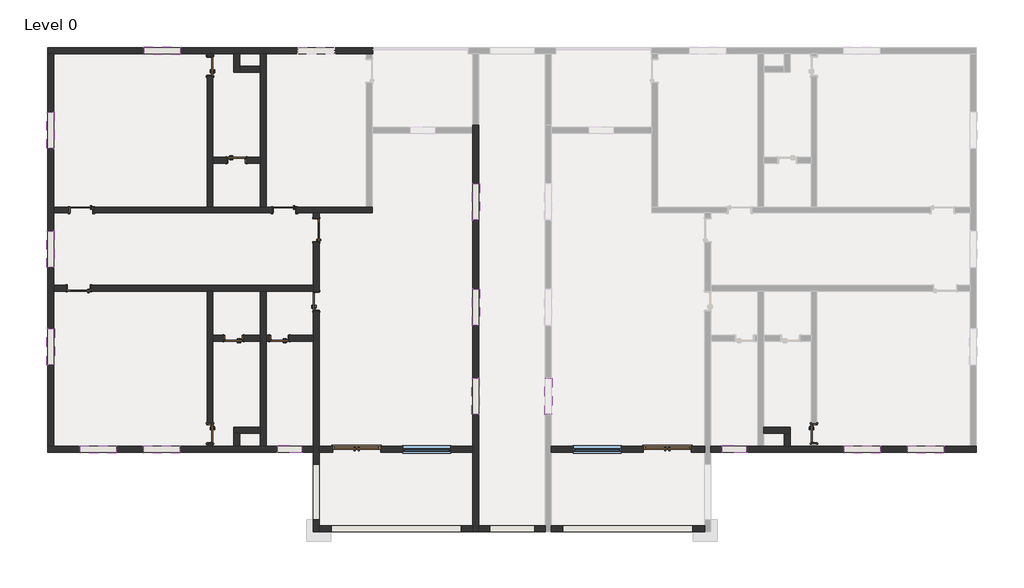
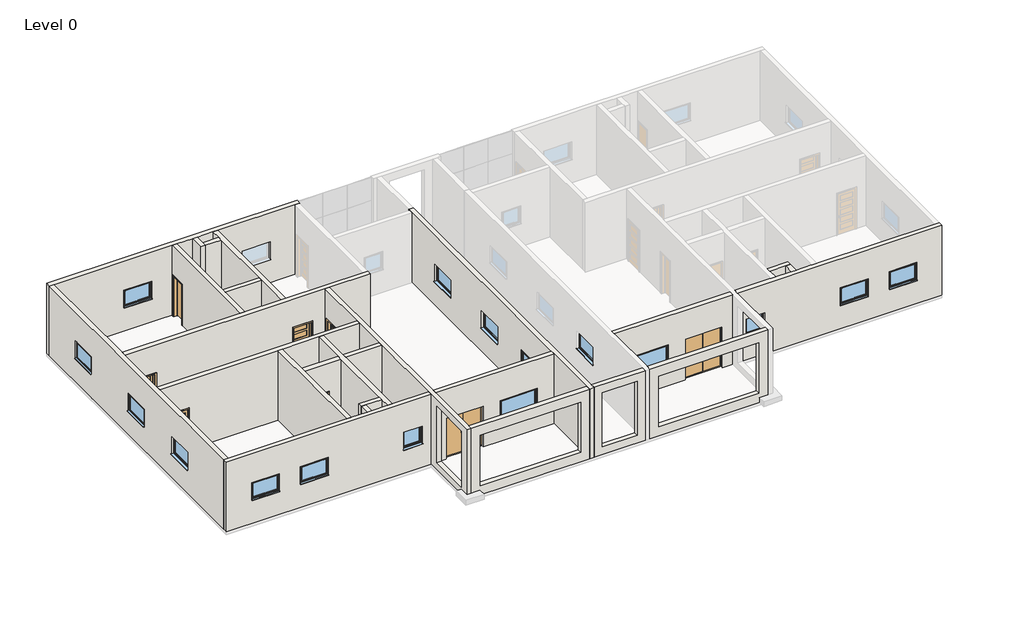
# One storey, part 1 of 2: 25 walls, 16 windows, 13 doors.
"""IFC4 building model written with IfcOpenShell, lengths in millimetres."""

from ifc_helpers import new_model, si_unit, frame, origin, origin_with_axes, place, context, project, spatial, polyline, outline, extrude, faceted_brep, transform, mapped, element, save
from components import door_interior_single_5_panel_vert_wood_door_interior_single_0f225555, door_interior_single_5_panel_vert_wood_door_interior_single_643f6a0b, doors_extdbl_flush_1810x2110mm_a954e790, doors_extdbl_flush_1810x2110mm_cf8af4c5, doors_intsgl_750x2110mm_542c0a28, doors_intsgl_750x2110mm_8b4efb5c, windows_sgl_plain_1360x910mm_f5b307ae, windows_sgl_plain_1360x910mm_8a2bb76a, windows_sgl_plain_1810x1210mm_77c2169a, windows_sgl_plain_1810x1210mm_541be4ad, windows_sgl_plain_910x910mm_7835b02d, windows_sgl_plain_910x910mm_23580505

model = new_model("IFC4")

# Units and contexts
model_context = context("Model", 3, world=origin())
ifc_project = project(units=[si_unit("LENGTHUNIT", "METRE", prefix="MILLI")], contexts=[model_context])

# Site, building, storey
site = spatial("IfcSite", under=ifc_project)
building = spatial("IfcBuilding", under=site)
storey = spatial("IfcBuildingStorey", under=building, Name="Level 0", Elevation=0.0)

# Doors
placement = place(None, origin())
door_interior_single_5_panel_vert_wood_door_interior_single_shape = door_interior_single_5_panel_vert_wood_door_interior_single_0f225555(model_context)
element("IfcDoor", 1, ObjectType="Door-Interior-Single-5_Panel_Vert-Wood : Door-Interior-Single-5_Panel_Vert-Wood", at=placement, inside=storey, context=model_context, shape_type="MappedRepresentation", body=[
    mapped(door_interior_single_5_panel_vert_wood_door_interior_single_shape, transform((-948.8269071, 3233.5358821, 0.0), x_axis=(-1.0, 0.0, 0.0), y_axis=(0.0, -1.0, 0.0), z_axis=(0.0, 0.0, 1.0))),
])
door_interior_single_5_panel_vert_wood_door_interior_single_2_shape = door_interior_single_5_panel_vert_wood_door_interior_single_643f6a0b(model_context)
element("IfcDoor", 2, ObjectType="Door-Interior-Single-5_Panel_Vert-Wood : Door-Interior-Single-5_Panel_Vert-Wood", at=placement, inside=storey, context=model_context, shape_type="MappedRepresentation", body=[
    mapped(door_interior_single_5_panel_vert_wood_door_interior_single_2_shape, transform((6788.6730929, 6189.8858821, 0.0), x_axis=(-1.0, 0.0, 0.0), y_axis=(0.0, -1.0, 0.0), z_axis=(0.0, 0.0, 1.0))),
])
element("IfcDoor", 3, ObjectType="Door-Interior-Single-5_Panel_Vert-Wood : Door-Interior-Single-5_Panel_Vert-Wood", at=placement, inside=storey, context=model_context, shape_type="MappedRepresentation", body=[
    mapped(door_interior_single_5_panel_vert_wood_door_interior_single_2_shape, transform((-848.8269071, 6189.8858821, 0.0), x_axis=(-1.0, 0.0, 0.0), y_axis=(0.0, -1.0, 0.0), z_axis=(0.0, 0.0, 1.0))),
])
element("IfcDoor", 4, ObjectType="Door-Interior-Single-5_Panel_Vert-Wood : Door-Interior-Single-5_Panel_Vert-Wood", at=placement, inside=storey, context=model_context, shape_type="MappedRepresentation", body=[
    mapped(door_interior_single_5_panel_vert_wood_door_interior_single_2_shape, transform((7991.8480929, 5424.2108821, 0.0), x_axis=(0.0, 1.0, 0.0), y_axis=(-1.0, 0.0, 0.0), z_axis=(0.0, 0.0, 1.0))),
])
doors_extdbl_flush_1810x2110mm_shape = doors_extdbl_flush_1810x2110mm_a954e790(model_context)
element("IfcDoor", 5, ObjectType="Doors_ExtDbl_Flush : 1810x2110mm", at=placement, inside=storey, context=model_context, shape_type="MappedRepresentation", body=[
    mapped(doors_extdbl_flush_1810x2110mm_shape, transform((9506.1730929, -2813.2891179, 0.0), x_axis=(1.0, 0.0, 0.0), y_axis=(0.0, 1.0, 0.0), z_axis=(0.0, 0.0, 1.0))),
])
doors_extdbl_flush_1810x2110mm_2_shape = doors_extdbl_flush_1810x2110mm_cf8af4c5(model_context)
element("IfcDoor", 6, ObjectType="Doors_ExtDbl_Flush : 1810x2110mm", at=placement, inside=storey, context=model_context, shape_type="MappedRepresentation", body=[
    mapped(doors_extdbl_flush_1810x2110mm_2_shape, transform((21196.1730929, -2813.2891179, 0.0), x_axis=(-1.0, 0.0, 0.0), y_axis=(0.0, -1.0, 0.0), z_axis=(0.0, 0.0, 1.0))),
])
doors_intsgl_750x2110mm_shape = doors_intsgl_750x2110mm_542c0a28(model_context)
element("IfcDoor", 7, ObjectType="Doors_IntSgl : 750x2110mm", at=placement, inside=storey, context=model_context, shape_type="MappedRepresentation", body=[
    mapped(doors_intsgl_750x2110mm_shape, transform((4988.6730929, 8061.7108821, 0.0), x_axis=(1.0, 0.0, 0.0), y_axis=(0.0, 1.0, 0.0), z_axis=(0.0, 0.0, 1.0))),
])
element("IfcDoor", 8, ObjectType="Doors_IntSgl : 750x2110mm", at=placement, inside=storey, context=model_context, shape_type="MappedRepresentation", body=[
    mapped(doors_intsgl_750x2110mm_shape, transform((4876.1730929, 1361.7108821, 0.0), x_axis=(-1.0, 0.0, 0.0), y_axis=(0.0, -1.0, 0.0), z_axis=(0.0, 0.0, 1.0))),
])
element("IfcDoor", 9, ObjectType="Doors_IntSgl : 750x2110mm", at=placement, inside=storey, context=model_context, shape_type="MappedRepresentation", body=[
    mapped(doors_intsgl_750x2110mm_shape, transform((6601.1730929, 1361.7108821, 0.0), x_axis=(-1.0, 0.0, 0.0), y_axis=(0.0, -1.0, 0.0), z_axis=(0.0, 0.0, 1.0))),
])
element("IfcDoor", 10, ObjectType="Doors_IntSgl : 750x2110mm", at=placement, inside=storey, context=model_context, shape_type="MappedRepresentation", body=[
    mapped(doors_intsgl_750x2110mm_shape, transform((7988.6730929, 2749.2108821, 0.0), x_axis=(0.0, 1.0, 0.0), y_axis=(-1.0, 0.0, 0.0), z_axis=(0.0, 0.0, 1.0))),
])
element("IfcDoor", 11, ObjectType="Doors_IntSgl : 750x2110mm", at=placement, inside=storey, context=model_context, shape_type="MappedRepresentation", body=[
    mapped(doors_intsgl_750x2110mm_shape, transform((3988.6730929, -2225.7891179, 0.0), x_axis=(0.0, -1.0, 0.0), y_axis=(1.0, 0.0, 0.0), z_axis=(0.0, 0.0, 1.0))),
])
doors_intsgl_750x2110mm_2_shape = doors_intsgl_750x2110mm_8b4efb5c(model_context)
element("IfcDoor", 12, ObjectType="Doors_IntSgl : 750x2110mm", at=placement, inside=storey, context=model_context, shape_type="MappedRepresentation", body=[
    mapped(doors_intsgl_750x2110mm_2_shape, transform((3988.6730929, 11599.2108821, 0.0), x_axis=(0.0, 1.0, 0.0), y_axis=(-1.0, 0.0, 0.0), z_axis=(0.0, 0.0, 1.0))),
])
element("IfcDoor", 13, ObjectType="Doors_IntSgl : 750x2110mm", at=placement, inside=storey, context=model_context, shape_type="MappedRepresentation", body=[
    mapped(doors_intsgl_750x2110mm_2_shape, transform((26713.6730929, -2225.7891179, 0.0), x_axis=(0.0, -1.0, 0.0), y_axis=(1.0, 0.0, 0.0), z_axis=(0.0, 0.0, 1.0))),
])

# Walls
element("IfcWall", 14, ObjectType="GENERIC 225", at=placement, inside=storey, context=model_context, shape_type="Brep", body=[
    faceted_brep([(-2123.8269071, 12074.2108821, 0.0), (-1898.8269071, 12074.2108821, 0.0), (3876.1730929, 12074.2108821, 0.0), (4101.1730929, 12074.2108821, 0.0), (4876.1730929, 12074.2108821, 0.0), (5101.1730929, 12074.2108821, 0.0), (5876.1730929, 12074.2108821, 0.0), (6101.1730929, 12074.2108821, 0.0), (9876.1730929, 12074.2108821, 0.0), (10101.1730929, 12074.2108821, 0.0), (10121.1730929, 12074.2108821, 0.0), (10121.1730929, 12074.2108821, 3600.0), (10101.1730929, 12074.2108821, 3600.0), (9876.1730929, 12074.2108821, 3600.0), (6101.1730929, 12074.2108821, 3600.0), (5876.1730929, 12074.2108821, 3600.0), (5101.1730929, 12074.2108821, 3600.0), (4876.1730929, 12074.2108821, 3600.0), (4101.1730929, 12074.2108821, 3600.0), (3876.1730929, 12074.2108821, 3600.0), (-1898.8269071, 12074.2108821, 3600.0), (-2123.8269071, 12074.2108821, 3600.0), (2876.1730929, 12074.2108821, 2110.0), (2876.1730929, 12074.2108821, 1200.0), (1516.1730929, 12074.2108821, 1200.0), (1516.1730929, 12074.2108821, 2110.0), (7308.6730929, 12074.2108821, 2110.0), (8668.6730929, 12074.2108821, 2110.0), (8668.6730929, 12074.2108821, 1200.0), (7308.6730929, 12074.2108821, 1200.0), (-2123.8269071, 12299.2108821, 0.0), (-2123.8269071, 12299.2108821, 3600.0), (10121.1730929, 12299.2108821, 3600.0), (10121.1730929, 12299.2108821, 0.0), (2876.1730929, 12299.2108821, 2110.0), (1516.1730929, 12299.2108821, 2110.0), (1516.1730929, 12299.2108821, 1200.0), (2876.1730929, 12299.2108821, 1200.0), (7308.6730929, 12299.2108821, 2110.0), (7308.6730929, 12299.2108821, 1200.0), (8668.6730929, 12299.2108821, 1200.0), (8668.6730929, 12299.2108821, 2110.0)], [[[0, 1, 2, 3, 4, 5, 6, 7, 8, 9, 10, 11, 12, 13, 14, 15, 16, 17, 18, 19, 20, 21], [22, 23, 24, 25], [26, 27, 28, 29]], [[30, 31, 32, 33], [34, 35, 36, 37], [38, 39, 40, 41]], [[10, 9, 8, 7, 6, 5, 4, 3, 2, 1, 0, 30, 33]], [[11, 10, 33, 32]], [[21, 20, 19, 18, 17, 16, 15, 14, 13, 12, 11, 32, 31]], [[0, 21, 31, 30]], [[23, 22, 34, 37]], [[24, 23, 37, 36]], [[25, 24, 36, 35]], [[22, 25, 35, 34]], [[39, 38, 26, 29]], [[40, 39, 29, 28]], [[41, 40, 28, 27]], [[38, 41, 27, 26]]]),
])
element("IfcWall", 15, ObjectType="GENERIC 225", at=placement, inside=storey, context=model_context, shape_type="Brep", body=[
    faceted_brep([(8101.1730929, 6074.2108821, 3600.0), (8101.1730929, -2700.7891179, 3600.0), (8101.1730929, -2925.7891179, 3600.0), (8101.1730929, -5700.7891179, 3600.0), (8101.1730929, -5925.7891179, 3600.0), (8101.1730929, -5925.7891179, 0.0), (8101.1730929, -5700.7891179, 0.0), (8101.1730929, -2925.7891179, 0.0), (8101.1730929, -2700.7891179, 0.0), (8101.1730929, 2374.2108821, 0.0), (8101.1730929, 2374.2108821, 2110.0), (8101.1730929, 3124.2108821, 2110.0), (8101.1730929, 3124.2108821, 0.0), (8101.1730929, 4974.2108821, 0.0), (8101.1730929, 4974.2108821, 2125.4), (8101.1730929, 5874.2108821, 2125.4), (8101.1730929, 5874.2108821, 0.0), (8101.1730929, 6074.2108821, 0.0), (8101.1730929, -5475.2269163, 3254.1937526), (8101.1730929, -3375.2269163, 3254.1937526), (8101.1730929, -3375.2269163, 354.1937526), (8101.1730929, -5475.2269163, 354.1937526), (7876.1730929, -5925.7891179, 3600.0), (7876.1730929, -2925.7891179, 3600.0), (7876.1730929, -2700.7891179, 3600.0), (7876.1730929, 1249.2108821, 3600.0), (7876.1730929, 1474.2108821, 3600.0), (7876.1730929, 3124.2108821, 3600.0), (7876.1730929, 3349.2108821, 3600.0), (7876.1730929, 6074.2108821, 3600.0), (7876.1730929, 6074.2108821, 0.0), (7876.1730929, 5874.2108821, 0.0), (7876.1730929, 5874.2108821, 2125.4), (7876.1730929, 4974.2108821, 2125.4), (7876.1730929, 4974.2108821, 0.0), (7876.1730929, 3349.2108821, 0.0), (7876.1730929, 3124.2108821, 0.0), (7876.1730929, 3124.2108821, 2110.0), (7876.1730929, 2374.2108821, 2110.0), (7876.1730929, 2374.2108821, 0.0), (7876.1730929, 1474.2108821, 0.0), (7876.1730929, 1249.2108821, 0.0), (7876.1730929, -2700.7891179, 0.0), (7876.1730929, -2925.7891179, 0.0), (7876.1730929, -5925.7891179, 0.0), (7876.1730929, -3375.2269163, 3254.1937526), (7876.1730929, -5475.2269163, 3254.1937526), (7876.1730929, -5475.2269163, 354.1937526), (7876.1730929, -3375.2269163, 354.1937526)], [[[0, 1, 2, 3, 4, 5, 6, 7, 8, 9, 10, 11, 12, 13, 14, 15, 16, 17], [18, 19, 20, 21]], [[22, 23, 24, 25, 26, 27, 28, 29, 30, 31, 32, 33, 34, 35, 36, 37, 38, 39, 40, 41, 42, 43, 44], [45, 46, 47, 48]], [[0, 17, 30, 29]], [[15, 32, 31, 16]], [[32, 15, 14, 33]], [[33, 14, 13, 34]], [[11, 37, 36, 12]], [[37, 11, 10, 38]], [[38, 10, 9, 39]], [[5, 4, 22, 44]], [[17, 16, 31, 30]], [[5, 44, 43, 42, 41, 40, 39, 9, 8, 7, 6]], [[34, 13, 12, 36, 35]], [[4, 3, 2, 1, 0, 29, 28, 27, 26, 25, 24, 23, 22]], [[19, 18, 46, 45]], [[20, 19, 45, 48]], [[21, 20, 48, 47]], [[18, 21, 47, 46]]]),
])
element("IfcWall", 16, ObjectType="GENERIC 225", at=placement, inside=storey, context=model_context, shape_type="Brep", body=[
    faceted_brep([(7876.1730929, -2700.7891179, 0.0), (6101.1730929, -2700.7891179, 0.0), (5876.1730929, -2700.7891179, 0.0), (5101.1730929, -2700.7891179, 0.0), (4876.1730929, -2700.7891179, 0.0), (4101.1730929, -2700.7891179, 0.0), (3876.1730929, -2700.7891179, 0.0), (-1898.8269071, -2700.7891179, 0.0), (-2123.8269071, -2700.7891179, 0.0), (-2123.8269071, -2700.7891179, 3600.0), (-1898.8269071, -2700.7891179, 3600.0), (3876.1730929, -2700.7891179, 3600.0), (4101.1730929, -2700.7891179, 3600.0), (4876.1730929, -2700.7891179, 3600.0), (5101.1730929, -2700.7891179, 3600.0), (5876.1730929, -2700.7891179, 3600.0), (6101.1730929, -2700.7891179, 3600.0), (7876.1730929, -2700.7891179, 3600.0), (461.1730929, -2700.7891179, 2110.0), (-898.8269071, -2700.7891179, 2110.0), (-898.8269071, -2700.7891179, 1200.0), (461.1730929, -2700.7891179, 1200.0), (2848.6730929, -2700.7891179, 2110.0), (1488.6730929, -2700.7891179, 2110.0), (1488.6730929, -2700.7891179, 1200.0), (2848.6730929, -2700.7891179, 1200.0), (6533.6730929, -2700.7891179, 2110.0), (6533.6730929, -2700.7891179, 1200.0), (7443.6730929, -2700.7891179, 1200.0), (7443.6730929, -2700.7891179, 2110.0), (7876.1730929, -2925.7891179, 0.0), (7876.1730929, -2925.7891179, 3600.0), (-2123.8269071, -2925.7891179, 3600.0), (-2123.8269071, -2925.7891179, 0.0), (461.1730929, -2925.7891179, 2110.0), (461.1730929, -2925.7891179, 1200.0), (-898.8269071, -2925.7891179, 1200.0), (-898.8269071, -2925.7891179, 2110.0), (2848.6730929, -2925.7891179, 2110.0), (2848.6730929, -2925.7891179, 1200.0), (1488.6730929, -2925.7891179, 1200.0), (1488.6730929, -2925.7891179, 2110.0), (6533.6730929, -2925.7891179, 2110.0), (7443.6730929, -2925.7891179, 2110.0), (7443.6730929, -2925.7891179, 1200.0), (6533.6730929, -2925.7891179, 1200.0)], [[[0, 1, 2, 3, 4, 5, 6, 7, 8, 9, 10, 11, 12, 13, 14, 15, 16, 17], [18, 19, 20, 21], [22, 23, 24, 25], [26, 27, 28, 29]], [[30, 31, 32, 33], [34, 35, 36, 37], [38, 39, 40, 41], [42, 43, 44, 45]], [[8, 7, 6, 5, 4, 3, 2, 1, 0, 30, 33]], [[17, 16, 15, 14, 13, 12, 11, 10, 9, 32, 31]], [[0, 17, 31, 30]], [[9, 8, 33, 32]], [[35, 34, 18, 21]], [[36, 35, 21, 20]], [[37, 36, 20, 19]], [[34, 37, 19, 18]], [[39, 38, 22, 25]], [[40, 39, 25, 24]], [[41, 40, 24, 23]], [[38, 41, 23, 22]], [[27, 26, 42, 45]], [[28, 27, 45, 44]], [[29, 28, 44, 43]], [[26, 29, 43, 42]]]),
])
element("IfcWall", 17, ObjectType="GENERIC 225", at=placement, inside=storey, context=model_context, shape_type="Brep", body=[
    faceted_brep([(-1898.8269071, -2700.7891179, 0.0), (-1898.8269071, 3124.2108821, 0.0), (-1898.8269071, 3349.2108821, 0.0), (-1898.8269071, 6074.2108821, 0.0), (-1898.8269071, 6299.2108821, 0.0), (-1898.8269071, 12074.2108821, 0.0), (-1898.8269071, 12074.2108821, 3600.0), (-1898.8269071, 6299.2108821, 3600.0), (-1898.8269071, 6074.2108821, 3600.0), (-1898.8269071, 3349.2108821, 3600.0), (-1898.8269071, 3124.2108821, 3600.0), (-1898.8269071, -2700.7891179, 3600.0), (-1898.8269071, 8506.7108821, 2110.0), (-1898.8269071, 9866.7108821, 2110.0), (-1898.8269071, 9866.7108821, 1200.0), (-1898.8269071, 8506.7108821, 1200.0), (-1898.8269071, 4031.7108821, 2110.0), (-1898.8269071, 5391.7108821, 2110.0), (-1898.8269071, 5391.7108821, 1200.0), (-1898.8269071, 4031.7108821, 1200.0), (-1898.8269071, 1724.2108821, 2110.0), (-1898.8269071, 1724.2108821, 1200.0), (-1898.8269071, 364.2108821, 1200.0), (-1898.8269071, 364.2108821, 2110.0), (-2123.8269071, -2700.7891179, 0.0), (-2123.8269071, -2700.7891179, 3600.0), (-2123.8269071, 12074.2108821, 3600.0), (-2123.8269071, 12074.2108821, 0.0), (-2123.8269071, 8506.7108821, 2110.0), (-2123.8269071, 8506.7108821, 1200.0), (-2123.8269071, 9866.7108821, 1200.0), (-2123.8269071, 9866.7108821, 2110.0), (-2123.8269071, 4031.7108821, 2110.0), (-2123.8269071, 4031.7108821, 1200.0), (-2123.8269071, 5391.7108821, 1200.0), (-2123.8269071, 5391.7108821, 2110.0), (-2123.8269071, 1724.2108821, 2110.0), (-2123.8269071, 364.2108821, 2110.0), (-2123.8269071, 364.2108821, 1200.0), (-2123.8269071, 1724.2108821, 1200.0)], [[[0, 1, 2, 3, 4, 5, 6, 7, 8, 9, 10, 11], [12, 13, 14, 15], [16, 17, 18, 19], [20, 21, 22, 23]], [[24, 25, 26, 27], [28, 29, 30, 31], [32, 33, 34, 35], [36, 37, 38, 39]], [[5, 4, 3, 2, 1, 0, 24, 27]], [[11, 10, 9, 8, 7, 6, 26, 25]], [[6, 5, 27, 26]], [[0, 11, 25, 24]], [[29, 28, 12, 15]], [[30, 29, 15, 14]], [[31, 30, 14, 13]], [[28, 31, 13, 12]], [[33, 32, 16, 19]], [[34, 33, 19, 18]], [[35, 34, 18, 17]], [[32, 35, 17, 16]], [[21, 20, 36, 39]], [[22, 21, 39, 38]], [[23, 22, 38, 37]], [[20, 23, 37, 36]]]),
])
element("IfcWall", 18, ObjectType="GENERIC 225", at=placement, inside=storey, context=model_context, shape_type="Brep", body=[
    faceted_brep([(7876.1730929, 3124.2108821, 3600.0), (6101.1730929, 3124.2108821, 3600.0), (5876.1730929, 3124.2108821, 3600.0), (4101.1730929, 3124.2108821, 3600.0), (3876.1730929, 3124.2108821, 3600.0), (-1898.8269071, 3124.2108821, 3600.0), (-1898.8269071, 3124.2108821, 0.0), (-1398.8269071, 3124.2108821, 0.0), (-1398.8269071, 3124.2108821, 2125.4), (-498.8269071, 3124.2108821, 2125.4), (-498.8269071, 3124.2108821, 0.0), (3876.1730929, 3124.2108821, 0.0), (4101.1730929, 3124.2108821, 0.0), (5876.1730929, 3124.2108821, 0.0), (6101.1730929, 3124.2108821, 0.0), (7876.1730929, 3124.2108821, 0.0), (7876.1730929, 3124.2108821, 2110.0), (-1898.8269071, 3349.2108821, 3600.0), (7876.1730929, 3349.2108821, 3600.0), (7876.1730929, 3349.2108821, 0.0), (-498.8269071, 3349.2108821, 0.0), (-498.8269071, 3349.2108821, 2125.4), (-1398.8269071, 3349.2108821, 2125.4), (-1398.8269071, 3349.2108821, 0.0), (-1898.8269071, 3349.2108821, 0.0)], [[[0, 1, 2, 3, 4, 5, 6, 7, 8, 9, 10, 11, 12, 13, 14, 15, 16]], [[17, 18, 19, 20, 21, 22, 23, 24]], [[6, 24, 23, 7]], [[19, 15, 14, 13, 12, 11, 10, 20]], [[5, 4, 3, 2, 1, 0, 18, 17]], [[6, 5, 17, 24]], [[0, 16, 15, 19, 18]], [[22, 8, 7, 23]], [[8, 22, 21, 9]], [[9, 21, 20, 10]]]),
])
element("IfcWall", 19, ObjectType="GENERIC 225", at=placement, inside=storey, context=model_context, shape_type="Brep", body=[
    faceted_brep([(3876.1730929, -2700.7891179, 3600.0), (3876.1730929, 3124.2108821, 3600.0), (3876.1730929, 3124.2108821, 0.0), (3876.1730929, -1850.7891179, 0.0), (3876.1730929, -1850.7891179, 2110.0), (3876.1730929, -2600.7891179, 2110.0), (3876.1730929, -2600.7891179, 0.0), (3876.1730929, -2700.7891179, 0.0), (4101.1730929, 3124.2108821, 3600.0), (4101.1730929, 1474.2108821, 3600.0), (4101.1730929, 1249.2108821, 3600.0), (4101.1730929, -2700.7891179, 3600.0), (4101.1730929, -2700.7891179, 0.0), (4101.1730929, -2600.7891179, 0.0), (4101.1730929, -2600.7891179, 2110.0), (4101.1730929, -1850.7891179, 2110.0), (4101.1730929, -1850.7891179, 0.0), (4101.1730929, 1249.2108821, 0.0), (4101.1730929, 1474.2108821, 0.0), (4101.1730929, 3124.2108821, 0.0)], [[[0, 1, 2, 3, 4, 5, 6, 7]], [[8, 9, 10, 11, 12, 13, 14, 15, 16, 17, 18, 19]], [[2, 19, 18, 17, 16, 3]], [[12, 7, 6, 13]], [[1, 0, 11, 10, 9, 8]], [[2, 1, 8, 19]], [[0, 7, 12, 11]], [[5, 14, 13, 6]], [[14, 5, 4, 15]], [[15, 4, 3, 16]]]),
])
element("IfcWall", 20, ObjectType="GENERIC 225", at=placement, inside=storey, context=model_context, shape_type="Brep", body=[
    faceted_brep([(10101.1730929, 6074.2108821, 3600.0), (8101.1730929, 6074.2108821, 3600.0), (7876.1730929, 6074.2108821, 3600.0), (-1898.8269071, 6074.2108821, 3600.0), (-1898.8269071, 6074.2108821, 0.0), (-1298.8269071, 6074.2108821, 0.0), (-1298.8269071, 6074.2108821, 2125.4), (-398.8269071, 6074.2108821, 2125.4), (-398.8269071, 6074.2108821, 0.0), (6338.6730929, 6074.2108821, 0.0), (6338.6730929, 6074.2108821, 2125.4), (7238.6730929, 6074.2108821, 2125.4), (7238.6730929, 6074.2108821, 0.0), (7876.1730929, 6074.2108821, 0.0), (8101.1730929, 6074.2108821, 0.0), (10101.1730929, 6074.2108821, 0.0), (-1898.8269071, 6299.2108821, 3600.0), (3876.1730929, 6299.2108821, 3600.0), (4101.1730929, 6299.2108821, 3600.0), (5876.1730929, 6299.2108821, 3600.0), (6101.1730929, 6299.2108821, 3600.0), (9876.1730929, 6299.2108821, 3600.0), (10101.1730929, 6299.2108821, 3600.0), (10101.1730929, 6299.2108821, 0.0), (9876.1730929, 6299.2108821, 0.0), (7238.6730929, 6299.2108821, 0.0), (7238.6730929, 6299.2108821, 2125.4), (6338.6730929, 6299.2108821, 2125.4), (6338.6730929, 6299.2108821, 0.0), (6101.1730929, 6299.2108821, 0.0), (5876.1730929, 6299.2108821, 0.0), (4101.1730929, 6299.2108821, 0.0), (3876.1730929, 6299.2108821, 0.0), (-398.8269071, 6299.2108821, 0.0), (-398.8269071, 6299.2108821, 2125.4), (-1298.8269071, 6299.2108821, 2125.4), (-1298.8269071, 6299.2108821, 0.0), (-1898.8269071, 6299.2108821, 0.0)], [[[0, 1, 2, 3, 4, 5, 6, 7, 8, 9, 10, 11, 12, 13, 14, 15]], [[16, 17, 18, 19, 20, 21, 22, 23, 24, 25, 26, 27, 28, 29, 30, 31, 32, 33, 34, 35, 36, 37]], [[4, 37, 36, 5]], [[23, 15, 14, 13, 12, 25, 24]], [[28, 9, 8, 33, 32, 31, 30, 29]], [[3, 2, 1, 0, 22, 21, 20, 19, 18, 17, 16]], [[4, 3, 16, 37]], [[0, 15, 23, 22]], [[10, 9, 28, 27]], [[11, 10, 27, 26]], [[12, 11, 26, 25]], [[35, 6, 5, 36]], [[6, 35, 34, 7]], [[7, 34, 33, 8]]]),
])
element("IfcWall", 21, ObjectType="GENERIC 225", at=placement, inside=storey, context=model_context, shape_type="Brep", body=[
    faceted_brep([(4101.1730929, 12074.2108821, 3600.0), (4101.1730929, 8174.2108821, 3600.0), (4101.1730929, 7949.2108821, 3600.0), (4101.1730929, 6299.2108821, 3600.0), (4101.1730929, 6299.2108821, 0.0), (4101.1730929, 7949.2108821, 0.0), (4101.1730929, 8174.2108821, 0.0), (4101.1730929, 11224.2108821, 0.0), (4101.1730929, 11224.2108821, 2110.0), (4101.1730929, 11974.2108821, 2110.0), (4101.1730929, 11974.2108821, 0.0), (4101.1730929, 12074.2108821, 0.0), (3876.1730929, 6299.2108821, 3600.0), (3876.1730929, 12074.2108821, 3600.0), (3876.1730929, 12074.2108821, 0.0), (3876.1730929, 11974.2108821, 0.0), (3876.1730929, 11974.2108821, 2110.0), (3876.1730929, 11224.2108821, 2110.0), (3876.1730929, 11224.2108821, 0.0), (3876.1730929, 6299.2108821, 0.0)], [[[0, 1, 2, 3, 4, 5, 6, 7, 8, 9, 10, 11]], [[12, 13, 14, 15, 16, 17, 18, 19]], [[4, 19, 18, 7, 6, 5]], [[14, 11, 10, 15]], [[3, 2, 1, 0, 13, 12]], [[4, 3, 12, 19]], [[0, 11, 14, 13]], [[9, 16, 15, 10]], [[16, 9, 8, 17]], [[17, 8, 7, 18]]]),
])
element("IfcWall", 22, ObjectType="GENERIC 225", at=placement, inside=storey, context=model_context, shape_type="Brep", body=[
    faceted_brep([(5876.1730929, 3124.2108821, 0.0), (5876.1730929, 1474.2108821, 0.0), (5876.1730929, 1249.2108821, 0.0), (5876.1730929, -1988.2891179, 0.0), (5876.1730929, -2213.2891179, 0.0), (5876.1730929, -2700.7891179, 0.0), (5876.1730929, -2700.7891179, 3600.0), (5876.1730929, -2213.2891179, 3600.0), (5876.1730929, -1988.2891179, 3600.0), (5876.1730929, 1249.2108821, 3600.0), (5876.1730929, 1474.2108821, 3600.0), (5876.1730929, 3124.2108821, 3600.0), (6101.1730929, 3124.2108821, 0.0), (6101.1730929, 3124.2108821, 3600.0), (6101.1730929, 1474.2108821, 3600.0), (6101.1730929, 1249.2108821, 3600.0), (6101.1730929, -2700.7891179, 3600.0), (6101.1730929, -2700.7891179, 0.0), (6101.1730929, 1249.2108821, 0.0), (6101.1730929, 1474.2108821, 0.0)], [[[0, 1, 2, 3, 4, 5, 6, 7, 8, 9, 10, 11]], [[12, 13, 14, 15, 16, 17, 18, 19]], [[5, 4, 3, 2, 1, 0, 12, 19, 18, 17]], [[11, 10, 9, 8, 7, 6, 16, 15, 14, 13]], [[6, 5, 17, 16]], [[0, 11, 13, 12]]]),
])
element("IfcWall", 23, ObjectType="GENERIC 225", at=placement, inside=storey, context=model_context, shape_type="Brep", body=[
    faceted_brep([(5876.1730929, 12074.2108821, 0.0), (5876.1730929, 11599.2108821, 0.0), (5876.1730929, 11374.2108821, 0.0), (5876.1730929, 8174.2108821, 0.0), (5876.1730929, 7949.2108821, 0.0), (5876.1730929, 6299.2108821, 0.0), (5876.1730929, 6299.2108821, 3600.0), (5876.1730929, 7949.2108821, 3600.0), (5876.1730929, 8174.2108821, 3600.0), (5876.1730929, 11374.2108821, 3600.0), (5876.1730929, 11599.2108821, 3600.0), (5876.1730929, 12074.2108821, 3600.0), (6101.1730929, 12074.2108821, 0.0), (6101.1730929, 12074.2108821, 3600.0), (6101.1730929, 6299.2108821, 3600.0), (6101.1730929, 6299.2108821, 0.0)], [[[0, 1, 2, 3, 4, 5, 6, 7, 8, 9, 10, 11]], [[12, 13, 14, 15]], [[5, 4, 3, 2, 1, 0, 12, 15]], [[11, 10, 9, 8, 7, 6, 14, 13]], [[0, 11, 13, 12]], [[6, 5, 15, 14]]]),
])
element("IfcWall", 24, ObjectType="GENERIC 225", at=placement, inside=storey, context=model_context, shape_type="SweptSolid", body=[
    extrude(outline(polyline([(3600.0, 5876.1730929), (3600.0, 4101.1730929), (0.0, 4101.1730929), (0.0, 4613.6730929), (2110.0, 4613.6730929), (2110.0, 5363.6730929), (0.0, 5363.6730929), (0.0, 5876.1730929), (3600.0, 5876.1730929)])), frame((0.0, 7949.2108821, 0.0), z_axis=(0.0, 1.0, 0.0), x_axis=(0.0, 0.0, 1.0)), (0.0, 0.0, 1.0), 225.0),
])
element("IfcWall", 25, ObjectType="GENERIC 225", at=placement, inside=storey, context=model_context, shape_type="SweptSolid", body=[
    extrude(outline(polyline([(0.0, 7876.1730929), (3600.0, 7876.1730929), (3600.0, 6101.1730929), (0.0, 6101.1730929), (0.0, 6226.1730929), (2110.0, 6226.1730929), (2110.0, 6976.1730929), (0.0, 6976.1730929), (0.0, 7876.1730929)])), frame((0.0, 1249.2108821, 0.0), z_axis=(0.0, 1.0, 0.0), x_axis=(0.0, 0.0, 1.0)), (0.0, 0.0, 1.0), 225.0),
    extrude(outline(polyline([(3600.0, 4101.1730929), (0.0, 4101.1730929), (0.0, 4501.1730929), (2110.0, 4501.1730929), (2110.0, 5251.1730929), (0.0, 5251.1730929), (0.0, 5876.1730929), (3600.0, 5876.1730929), (3600.0, 4101.1730929)])), frame((0.0, 1249.2108821, 0.0), z_axis=(0.0, 1.0, 0.0), x_axis=(0.0, 0.0, 1.0)), (0.0, 0.0, 1.0), 225.0),
])
element("IfcWall", 26, ObjectType="GENERIC 225", at=placement, inside=storey, context=model_context, shape_type="SweptSolid", body=[
    extrude(outline(polyline([(2110.0, 10411.1730929), (0.0, 10411.1730929), (0.0, 13876.1730929), (3600.0, 13876.1730929), (3600.0, 8101.1730929), (0.0, 8101.1730929), (0.0, 8601.1730929), (2110.0, 8601.1730929), (2110.0, 10411.1730929)]), holes=[polyline([(2110.0, 13048.6730929), (900.0, 13048.6730929), (900.0, 11238.6730929), (2110.0, 11238.6730929), (2110.0, 13048.6730929)])]), frame((0.0, -2925.7891179, 0.0), z_axis=(0.0, 1.0, 0.0), x_axis=(0.0, 0.0, 1.0)), (0.0, 0.0, 1.0), 225.0),
])
element("IfcWall", 27, ObjectType="GENERIC 225", at=placement, inside=storey, context=model_context, shape_type="Brep", body=[
    faceted_brep([(5876.1730929, -1988.2891179, 0.0), (4876.1730929, -1988.2891179, 0.0), (4876.1730929, -1988.2891179, 3600.0), (5876.1730929, -1988.2891179, 3600.0), (5876.1730929, -2213.2891179, 0.0), (5876.1730929, -2213.2891179, 3600.0), (5101.1730929, -2213.2891179, 3600.0), (4876.1730929, -2213.2891179, 3600.0), (4876.1730929, -2213.2891179, 0.0), (5101.1730929, -2213.2891179, 0.0)], [[[0, 1, 2, 3]], [[4, 5, 6, 7, 8, 9]], [[1, 0, 4, 9, 8]], [[3, 2, 7, 6, 5]], [[0, 3, 5, 4]], [[2, 1, 8, 7]]]),
])
element("IfcWall", 28, ObjectType="GENERIC 225", at=placement, inside=storey, context=model_context, shape_type="SweptSolid", body=[
    extrude(outline(polyline([(4876.1730929, -2700.7891179), (4876.1730929, -2213.2891179), (5101.1730929, -2213.2891179), (5101.1730929, -2700.7891179), (4876.1730929, -2700.7891179)])), origin_with_axes(), (0.0, 0.0, 1.0), 3600.0),
])
element("IfcWall", 29, ObjectType="GENERIC 225", at=placement, inside=storey, context=model_context, shape_type="Brep", body=[
    faceted_brep([(4876.1730929, 12074.2108821, 0.0), (4876.1730929, 11374.2108821, 0.0), (4876.1730929, 11374.2108821, 3600.0), (4876.1730929, 12074.2108821, 3600.0), (5101.1730929, 12074.2108821, 0.0), (5101.1730929, 12074.2108821, 3600.0), (5101.1730929, 11599.2108821, 3600.0), (5101.1730929, 11374.2108821, 3600.0), (5101.1730929, 11374.2108821, 0.0), (5101.1730929, 11599.2108821, 0.0)], [[[0, 1, 2, 3]], [[4, 5, 6, 7, 8, 9]], [[1, 0, 4, 9, 8]], [[3, 2, 7, 6, 5]], [[0, 3, 5, 4]], [[2, 1, 8, 7]]]),
])
element("IfcWall", 30, ObjectType="GENERIC 225", at=placement, inside=storey, context=model_context, shape_type="SweptSolid", body=[
    extrude(outline(polyline([(5876.1730929, 11374.2108821), (5101.1730929, 11374.2108821), (5101.1730929, 11599.2108821), (5876.1730929, 11599.2108821), (5876.1730929, 11374.2108821)])), origin_with_axes(), (0.0, 0.0, 1.0), 3600.0),
])
element("IfcWall", 31, ObjectType="GENERIC 225", at=placement, inside=storey, context=model_context, shape_type="Brep", body=[
    faceted_brep([(13876.1730929, 9374.2108821, 0.0), (13876.1730929, 9299.2108821, 0.0), (13876.1730929, 9074.2108821, 0.0), (13876.1730929, -2700.7891179, 0.0), (13876.1730929, -2925.7891179, 0.0), (13876.1730929, -5700.7891179, 0.0), (13876.1730929, -5925.7891179, 0.0), (13876.1730929, -5925.7891179, 3600.0), (13876.1730929, -5700.7891179, 3600.0), (13876.1730929, -2925.7891179, 3600.0), (13876.1730929, -2700.7891179, 3600.0), (13876.1730929, 9074.2108821, 3600.0), (13876.1730929, 9299.2108821, 3600.0), (13876.1730929, 9374.2108821, 3600.0), (13876.1730929, 7174.2108821, 2110.0), (13876.1730929, 5814.2108821, 2110.0), (13876.1730929, 5814.2108821, 1200.0), (13876.1730929, 7174.2108821, 1200.0), (13876.1730929, 3214.2108821, 2110.0), (13876.1730929, 1854.2108821, 2110.0), (13876.1730929, 1854.2108821, 1200.0), (13876.1730929, 3214.2108821, 1200.0), (13876.1730929, -1500.7891179, 2110.0), (13876.1730929, -1500.7891179, 1200.0), (13876.1730929, -140.7891179, 1200.0), (13876.1730929, -140.7891179, 2110.0), (14101.1730929, 9374.2108821, 0.0), (14101.1730929, 9374.2108821, 3600.0), (14101.1730929, -5700.7891179, 3600.0), (14101.1730929, -5925.7891179, 3600.0), (14101.1730929, -5925.7891179, 0.0), (14101.1730929, -5700.7891179, 0.0), (14101.1730929, 7174.2108821, 2110.0), (14101.1730929, 7174.2108821, 1200.0), (14101.1730929, 5814.2108821, 1200.0), (14101.1730929, 5814.2108821, 2110.0), (14101.1730929, 3214.2108821, 2110.0), (14101.1730929, 3214.2108821, 1200.0), (14101.1730929, 1854.2108821, 1200.0), (14101.1730929, 1854.2108821, 2110.0), (14101.1730929, -1500.7891179, 2110.0), (14101.1730929, -140.7891179, 2110.0), (14101.1730929, -140.7891179, 1200.0), (14101.1730929, -1500.7891179, 1200.0)], [[[0, 1, 2, 3, 4, 5, 6, 7, 8, 9, 10, 11, 12, 13], [14, 15, 16, 17], [18, 19, 20, 21], [22, 23, 24, 25]], [[26, 27, 28, 29, 30, 31], [32, 33, 34, 35], [36, 37, 38, 39], [40, 41, 42, 43]], [[6, 5, 4, 3, 2, 1, 0, 26, 31, 30]], [[13, 12, 11, 10, 9, 8, 7, 29, 28, 27]], [[0, 13, 27, 26]], [[32, 35, 15, 14]], [[35, 34, 16, 15]], [[34, 33, 17, 16]], [[33, 32, 14, 17]], [[36, 39, 19, 18]], [[39, 38, 20, 19]], [[38, 37, 21, 20]], [[37, 36, 18, 21]], [[22, 25, 41, 40]], [[25, 24, 42, 41]], [[24, 23, 43, 42]], [[23, 22, 40, 43]], [[7, 6, 30, 29]]]),
])
element("IfcWall", 32, ObjectType="GENERIC 225", at=placement, inside=storey, context=model_context, shape_type="SweptSolid", body=[
    extrude(outline(polyline([(0.0, 8101.1730929), (0.0, 13876.1730929), (3600.0, 13876.1730929), (3600.0, 8101.1730929), (0.0, 8101.1730929)]), holes=[polyline([(3078.4755262, 13448.3751977), (478.4755262, 13448.3751977), (478.4755262, 8548.3751977), (3078.4755262, 8548.3751977), (3078.4755262, 13448.3751977)])]), frame((0.0, -5925.7891179, 0.0), z_axis=(0.0, 1.0, 0.0), x_axis=(0.0, 0.0, 1.0)), (0.0, 0.0, 1.0), 225.0),
])
element("IfcWall", 33, ObjectType="GENERIC 225", at=placement, inside=storey, context=model_context, shape_type="Brep", body=[
    faceted_brep([(22826.1730929, -2925.7891179, 0.0), (32826.1730929, -2925.7891179, 0.0), (32826.1730929, -2925.7891179, 3600.0), (22826.1730929, -2925.7891179, 3600.0), (30241.1730929, -2925.7891179, 2110.0), (31601.1730929, -2925.7891179, 2110.0), (31601.1730929, -2925.7891179, 1200.0), (30241.1730929, -2925.7891179, 1200.0), (27853.6730929, -2925.7891179, 2110.0), (29213.6730929, -2925.7891179, 2110.0), (29213.6730929, -2925.7891179, 1200.0), (27853.6730929, -2925.7891179, 1200.0), (24168.6730929, -2925.7891179, 2110.0), (24168.6730929, -2925.7891179, 1200.0), (23258.6730929, -2925.7891179, 1200.0), (23258.6730929, -2925.7891179, 2110.0), (22826.1730929, -2700.7891179, 0.0), (22826.1730929, -2700.7891179, 3600.0), (24601.1730929, -2700.7891179, 3600.0), (24826.1730929, -2700.7891179, 3600.0), (25601.1730929, -2700.7891179, 3600.0), (25826.1730929, -2700.7891179, 3600.0), (26601.1730929, -2700.7891179, 3600.0), (26826.1730929, -2700.7891179, 3600.0), (32601.1730929, -2700.7891179, 3600.0), (32826.1730929, -2700.7891179, 3600.0), (32826.1730929, -2700.7891179, 0.0), (32601.1730929, -2700.7891179, 0.0), (26826.1730929, -2700.7891179, 0.0), (26601.1730929, -2700.7891179, 0.0), (25826.1730929, -2700.7891179, 0.0), (25601.1730929, -2700.7891179, 0.0), (24826.1730929, -2700.7891179, 0.0), (24601.1730929, -2700.7891179, 0.0), (30241.1730929, -2700.7891179, 2110.0), (30241.1730929, -2700.7891179, 1200.0), (31601.1730929, -2700.7891179, 1200.0), (31601.1730929, -2700.7891179, 2110.0), (27853.6730929, -2700.7891179, 2110.0), (27853.6730929, -2700.7891179, 1200.0), (29213.6730929, -2700.7891179, 1200.0), (29213.6730929, -2700.7891179, 2110.0), (24168.6730929, -2700.7891179, 2110.0), (23258.6730929, -2700.7891179, 2110.0), (23258.6730929, -2700.7891179, 1200.0), (24168.6730929, -2700.7891179, 1200.0)], [[[0, 1, 2, 3], [4, 5, 6, 7], [8, 9, 10, 11], [12, 13, 14, 15]], [[16, 17, 18, 19, 20, 21, 22, 23, 24, 25, 26, 27, 28, 29, 30, 31, 32, 33], [34, 35, 36, 37], [38, 39, 40, 41], [42, 43, 44, 45]], [[1, 0, 16, 33, 32, 31, 30, 29, 28, 27, 26]], [[3, 2, 25, 24, 23, 22, 21, 20, 19, 18, 17]], [[0, 3, 17, 16]], [[2, 1, 26, 25]], [[35, 34, 4, 7]], [[36, 35, 7, 6]], [[37, 36, 6, 5]], [[34, 37, 5, 4]], [[39, 38, 8, 11]], [[40, 39, 11, 10]], [[41, 40, 10, 9]], [[38, 41, 9, 8]], [[13, 12, 42, 45]], [[14, 13, 45, 44]], [[15, 14, 44, 43]], [[12, 15, 43, 42]]]),
])
element("IfcWall", 34, ObjectType="GENERIC 225", at=placement, inside=storey, context=model_context, shape_type="SweptSolid", body=[
    extrude(outline(polyline([(0.0, 16826.1730929), (0.0, 20291.1730929), (2110.0, 20291.1730929), (2110.0, 22101.1730929), (0.0, 22101.1730929), (0.0, 22601.1730929), (3600.0, 22601.1730929), (3600.0, 16826.1730929), (0.0, 16826.1730929)]), holes=[polyline([(2110.0, 17653.6730929), (2110.0, 19463.6730929), (900.0, 19463.6730929), (900.0, 17653.6730929), (2110.0, 17653.6730929)])]), frame((0.0, -2925.7891179, 0.0), z_axis=(0.0, 1.0, 0.0), x_axis=(0.0, 0.0, 1.0)), (0.0, 0.0, 1.0), 225.0),
])
element("IfcWall", 35, ObjectType="GENERIC 225", at=placement, inside=storey, context=model_context, shape_type="Brep", body=[
    faceted_brep([(24826.1730929, -2213.2891179, 0.0), (25601.1730929, -2213.2891179, 0.0), (25826.1730929, -2213.2891179, 0.0), (25826.1730929, -2213.2891179, 3600.0), (25601.1730929, -2213.2891179, 3600.0), (24826.1730929, -2213.2891179, 3600.0), (24826.1730929, -1988.2891179, 0.0), (24826.1730929, -1988.2891179, 3600.0), (25826.1730929, -1988.2891179, 3600.0), (25826.1730929, -1988.2891179, 0.0)], [[[0, 1, 2, 3, 4, 5]], [[6, 7, 8, 9]], [[2, 1, 0, 6, 9]], [[5, 4, 3, 8, 7]], [[0, 5, 7, 6]], [[3, 2, 9, 8]]]),
])
element("IfcWall", 36, ObjectType="GENERIC 225", at=placement, inside=storey, context=model_context, shape_type="SweptSolid", body=[
    extrude(outline(polyline([(25601.1730929, -2700.7891179), (25601.1730929, -2213.2891179), (25826.1730929, -2213.2891179), (25826.1730929, -2700.7891179), (25601.1730929, -2700.7891179)])), origin_with_axes(), (0.0, 0.0, 1.0), 3600.0),
])
element("IfcWall", 37, ObjectType="GENERIC 225", at=placement, inside=storey, context=model_context, shape_type="SweptSolid", body=[
    extrude(outline(polyline([(0.0, 22601.1730929), (3600.0, 22601.1730929), (3600.0, 16826.1730929), (0.0, 16826.1730929), (0.0, 22601.1730929)]), holes=[polyline([(3078.4755262, 17253.970988), (3078.4755262, 22153.970988), (478.4755262, 22153.970988), (478.4755262, 17253.970988), (3078.4755262, 17253.970988)])]), frame((0.0, -5925.7891179, 0.0), z_axis=(0.0, 1.0, 0.0), x_axis=(0.0, 0.0, 1.0)), (0.0, 0.0, 1.0), 225.0),
])
element("IfcWall", 38, ObjectType="GENERIC 225", at=placement, inside=storey, context=model_context, shape_type="SweptSolid", body=[
    extrude(outline(polyline([(3600.0, 14101.1730929), (0.0, 14101.1730929), (0.0, 16601.1730929), (3600.0, 16601.1730929), (3600.0, 14101.1730929)]), holes=[polyline([(3195.6109116, 16206.6288359), (395.6109116, 16206.6288359), (395.6109116, 14506.6288359), (3195.6109116, 14506.6288359), (3195.6109116, 16206.6288359)])]), frame((0.0, -5925.7891179, 0.0), z_axis=(0.0, 1.0, 0.0), x_axis=(0.0, 0.0, 1.0)), (0.0, 0.0, 1.0), 225.0),
])

# Windows
windows_sgl_plain_1360x910mm_shape = windows_sgl_plain_1360x910mm_f5b307ae(model_context)
element("IfcWindow", 39, ObjectType="Windows_Sgl_Plain : 1360x910mm", at=placement, inside=storey, context=model_context, shape_type="MappedRepresentation", body=[
    mapped(windows_sgl_plain_1360x910mm_shape, transform((2196.1730929, 12195.16745, 0.0), x_axis=(-1.0, 0.0, 0.0), y_axis=(0.0, -1.0, 0.0), z_axis=(0.0, 0.0, 1.0))),
])
element("IfcWindow", 40, ObjectType="Windows_Sgl_Plain : 1360x910mm", at=placement, inside=storey, context=model_context, shape_type="MappedRepresentation", body=[
    mapped(windows_sgl_plain_1360x910mm_shape, transform((-2002.8703393, 9186.7108821, 0.0), x_axis=(0.0, 1.0, 0.0), y_axis=(-1.0, 0.0, 0.0), z_axis=(0.0, 0.0, 1.0))),
])
element("IfcWindow", 41, ObjectType="Windows_Sgl_Plain : 1360x910mm", at=placement, inside=storey, context=model_context, shape_type="MappedRepresentation", body=[
    mapped(windows_sgl_plain_1360x910mm_shape, transform((-2002.8703393, 4711.7108821, 0.0), x_axis=(0.0, 1.0, 0.0), y_axis=(-1.0, 0.0, 0.0), z_axis=(0.0, 0.0, 1.0))),
])
element("IfcWindow", 42, ObjectType="Windows_Sgl_Plain : 1360x910mm", at=placement, inside=storey, context=model_context, shape_type="MappedRepresentation", body=[
    mapped(windows_sgl_plain_1360x910mm_shape, transform((-2019.783475, 1044.2108821, 0.0), x_axis=(0.0, -1.0, 0.0), y_axis=(1.0, 0.0, 0.0), z_axis=(0.0, 0.0, 1.0))),
])
element("IfcWindow", 43, ObjectType="Windows_Sgl_Plain : 1360x910mm", at=placement, inside=storey, context=model_context, shape_type="MappedRepresentation", body=[
    mapped(windows_sgl_plain_1360x910mm_shape, transform((-218.8269071, -2804.83255, 0.0), x_axis=(-1.0, 0.0, 0.0), y_axis=(0.0, -1.0, 0.0), z_axis=(0.0, 0.0, 1.0))),
])
element("IfcWindow", 44, ObjectType="Windows_Sgl_Plain : 1360x910mm", at=placement, inside=storey, context=model_context, shape_type="MappedRepresentation", body=[
    mapped(windows_sgl_plain_1360x910mm_shape, transform((2168.6730929, -2804.83255, 0.0), x_axis=(-1.0, 0.0, 0.0), y_axis=(0.0, -1.0, 0.0), z_axis=(0.0, 0.0, 1.0))),
])
element("IfcWindow", 45, ObjectType="Windows_Sgl_Plain : 1360x910mm", at=placement, inside=storey, context=model_context, shape_type="MappedRepresentation", body=[
    mapped(windows_sgl_plain_1360x910mm_shape, transform((13980.216525, 6494.2108821, 0.0), x_axis=(0.0, -1.0, 0.0), y_axis=(1.0, 0.0, 0.0), z_axis=(0.0, 0.0, 1.0))),
])
element("IfcWindow", 46, ObjectType="Windows_Sgl_Plain : 1360x910mm", at=placement, inside=storey, context=model_context, shape_type="MappedRepresentation", body=[
    mapped(windows_sgl_plain_1360x910mm_shape, transform((13980.216525, 2534.2108821, 0.0), x_axis=(0.0, -1.0, 0.0), y_axis=(1.0, 0.0, 0.0), z_axis=(0.0, 0.0, 1.0))),
])
element("IfcWindow", 47, ObjectType="Windows_Sgl_Plain : 1360x910mm", at=placement, inside=storey, context=model_context, shape_type="MappedRepresentation", body=[
    mapped(windows_sgl_plain_1360x910mm_shape, transform((13997.1296607, -820.7891179, 0.0), x_axis=(0.0, 1.0, 0.0), y_axis=(-1.0, 0.0, 0.0), z_axis=(0.0, 0.0, 1.0))),
])
windows_sgl_plain_1360x910mm_2_shape = windows_sgl_plain_1360x910mm_8a2bb76a(model_context)
element("IfcWindow", 48, ObjectType="Windows_Sgl_Plain : 1360x910mm", at=placement, inside=storey, context=model_context, shape_type="MappedRepresentation", body=[
    mapped(windows_sgl_plain_1360x910mm_2_shape, transform((30921.1730929, -2804.83255, 0.0), x_axis=(1.0, 0.0, 0.0), y_axis=(0.0, 1.0, 0.0), z_axis=(0.0, 0.0, 1.0))),
])
element("IfcWindow", 49, ObjectType="Windows_Sgl_Plain : 1360x910mm", at=placement, inside=storey, context=model_context, shape_type="MappedRepresentation", body=[
    mapped(windows_sgl_plain_1360x910mm_2_shape, transform((28533.6730929, -2804.83255, 0.0), x_axis=(1.0, 0.0, 0.0), y_axis=(0.0, 1.0, 0.0), z_axis=(0.0, 0.0, 1.0))),
])
element("IfcWindow", 50, ObjectType="Windows_Sgl_Plain : 1360x910mm", at=placement, inside=storey, context=model_context, shape_type="MappedRepresentation", body=[
    mapped(windows_sgl_plain_1360x910mm_2_shape, transform((16705.216525, -820.7891179, 0.0), x_axis=(0.0, 1.0, 0.0), y_axis=(-1.0, 0.0, 0.0), z_axis=(0.0, 0.0, 1.0))),
])
windows_sgl_plain_1810x1210mm_shape = windows_sgl_plain_1810x1210mm_77c2169a(model_context)
element("IfcWindow", 51, ObjectType="Windows_Sgl_Plain : 1810x1210mm", at=placement, inside=storey, context=model_context, shape_type="MappedRepresentation", body=[
    mapped(windows_sgl_plain_1810x1210mm_shape, transform((12143.6730929, -2804.83255, 0.0), x_axis=(-1.0, 0.0, 0.0), y_axis=(0.0, -1.0, 0.0), z_axis=(0.0, 0.0, 1.0))),
])
windows_sgl_plain_1810x1210mm_2_shape = windows_sgl_plain_1810x1210mm_541be4ad(model_context)
element("IfcWindow", 52, ObjectType="Windows_Sgl_Plain : 1810x1210mm", at=placement, inside=storey, context=model_context, shape_type="MappedRepresentation", body=[
    mapped(windows_sgl_plain_1810x1210mm_2_shape, transform((18558.6730929, -2804.83255, 0.0), x_axis=(1.0, 0.0, 0.0), y_axis=(0.0, 1.0, 0.0), z_axis=(0.0, 0.0, 1.0))),
])
windows_sgl_plain_910x910mm_shape = windows_sgl_plain_910x910mm_7835b02d(model_context)
element("IfcWindow", 53, ObjectType="Windows_Sgl_Plain : 910x910mm", at=placement, inside=storey, context=model_context, shape_type="MappedRepresentation", body=[
    mapped(windows_sgl_plain_910x910mm_shape, transform((6988.6730929, -2821.7456857, 0.0), x_axis=(1.0, 0.0, 0.0), y_axis=(0.0, 1.0, 0.0), z_axis=(0.0, 0.0, 1.0))),
])
windows_sgl_plain_910x910mm_2_shape = windows_sgl_plain_910x910mm_23580505(model_context)
element("IfcWindow", 54, ObjectType="Windows_Sgl_Plain : 910x910mm", at=placement, inside=storey, context=model_context, shape_type="MappedRepresentation", body=[
    mapped(windows_sgl_plain_910x910mm_2_shape, transform((23713.6730929, -2821.7456857, 0.0), x_axis=(-1.0, 0.0, 0.0), y_axis=(0.0, -1.0, 0.0), z_axis=(0.0, 0.0, 1.0))),
])

save(model, "model.ifc")

# Revit data of these elements
# Grids (mm)
#   "13": line (7988.673, -8390.349) -> (7988.673, 18334.57)
#   "5": line (38979.424, 6186.711) -> (-6202.184, 6186.711)
#   "6": line (38979.424, 9186.711) -> (-6202.184, 9186.711)
#   "7": line (38979.424, 12186.711) -> (-6202.184, 12186.711)
#   "8": line (-2011.327, -8390.349) -> (-2011.327, 18334.57)
#   "9": line (-11.327, -8390.349) -> (-11.327, 18334.57)
#   "10": line (1988.673, -8390.349) -> (1988.673, 18334.57)
#   "11": line (3988.673, -8390.349) -> (3988.673, 18334.57)
#   "12": line (5988.673, -8390.349) -> (5988.673, 18334.57)
#   "14": line (9988.673, -8390.349) -> (9988.673, 18334.57)
#   "17": line (15988.673, -8390.349) -> (15988.673, 18334.57)
#   "18": line (17988.673, -8390.349) -> (17988.673, 18334.57)
#   "19": line (19988.673, -8390.349) -> (19988.673, 18334.57)
#   "20": line (21988.673, -8390.349) -> (21988.673, 18334.57)
#   "15": line (11988.673, -8390.349) -> (11988.673, 18334.57)
#   "16": line (13988.673, -8390.349) -> (13988.673, 18334.57)
#   "25": line (31988.673, -8390.349) -> (31988.673, 18334.57)
#   "21": line (23988.673, -8390.349) -> (23988.673, 18334.57)
#   "22": line (25988.673, -8390.349) -> (25988.673, 18334.57)
#   "23": line (27988.673, -8390.349) -> (27988.673, 18334.57)
#   "24": line (29988.673, -8390.349) -> (29988.673, 18334.57)
#   "26": line (33988.673, -8390.349) -> (33988.673, 18334.57)
#   "27": line (35988.673, -8390.349) -> (35988.673, 18334.57)
#   "3": line (38979.424, 186.711) -> (-6202.184, 186.711)
#   "1": line (38979.424, -5813.289) -> (-6202.184, -5813.289)
#   "2": line (38979.424, -2813.289) -> (-6202.184, -2813.289)
#   "4": line (38979.424, 3186.711) -> (-6202.184, 3186.711)
# Type "Door-Interior-Single-5_Panel_Vert-Wood : Door-Interior-Single-5_Panel_Vert-Wood"
#   Type Mark = "46"
#   Assembly Code = "C1020300"
#   Analytic Construction = "Wooden"
#   Top Rail = 119.063 mm
#   Thickness = 34.925 mm
#   Thermal Resistance (R) = 0.455703 (m²·K)/W
#   Swing Angle [instance default] = 90.00°
#   Stiles = 120.65 mm
#   Rough Width = 900 mm
#   Rough Height = 2125.4 mm
#   Intermediate Rail = 114.3 mm
#   Height = 2100 mm
#   Width = 849.2 mm
#   Heat Transfer Coefficient (U) = 2.19465 W/(m²·K)
#   Bottom Rail = 231.775 mm
#   Trim Material = Cherry
#   Panel Material = Cherry
#   Frame Material = Cherry
#   Door Handle Material = Aluminum
#   Visual Light Transmittance = 0
#   Solar Heat Gain Coefficient = 0
#   Wall Closure = (empty or 0)
#   Function = (empty or 0)
# Type "Doors_ExtDbl_Flush : 1810x2110mm"
#   Type Mark = "44"
#   Type Comments = "External Double"
#   Operation = "DoubleDoorSingleSwing"
#   Keynote = "L20"
#   Analytic Construction = "Metal"
#   Wrap Layers (Ext) from Ext = 102.5 mm
#   Wrap Layers (Int) from Ext = 177.5 mm
#   Thickness = 44 mm
#   Rough Width = 1810 mm
#   Rough Height = 2110 mm
#   O/A Frame Width = 64 mm
#   Heat Transfer Coefficient (U) = 3.7021 W/(m²·K)
#   Handle Z Distance = 1050 mm
#   FrameWidth = 42 mm
#   FrameOffset - External = 25 mm
#   FrameDepth = 89 mm
#   Door Panel Width = 852 mm
#   Door Panel Thickness = 44 mm
#   Door Panel Height = 2000 mm
#   Cill Thickness = 54.5 mm
#   Cill Projection = 30 mm
#   Handle X Distance = 75 mm
#   Height = 2110 mm
#   Structural Tolerance = 6.5 mm
#   Tolerance = 3 mm
#   Undercut = 4 mm
#   Width = 1810 mm
#   Cill Extension = 25 mm
#   Cavity Closer Width = 50 mm
#   Cavity Closer Offset from Ext = 102.5 mm
#   Cavity Closer Depth = 85 mm
#   Define Thermal Properties by = 0
#   Vis - Ironmongery = yes
#   Vis - Cavity Closers = yes
#   Function = 1
#   Material Door = Door - Panel
#   Material Frame = Door - Frame/Mullion
#   Material Ironmongery = Door - Handle
#   Visual Light Transmittance = 0
#   Thermal Resistance (R) = 0
#   Solar Heat Gain Coefficient = 0
#   Wall Closure = (empty or 0)
# Type "Doors_IntSgl : 750x2110mm"
#   Construction Type Id = "MDOOR"
#   Type Mark = "42"
#   Type Comments = "Internal Single"
#   Operation = "SingleSwingRight"
#   Manufacturer = "Revit"
#   Keynote = "L20"
#   Description = "Internal Single Door"
#   Analytic Construction = "Metal"
#   UnderCut = 8 mm
#   Tolerance = 2 mm
#   Thickness = 38 mm
#   Thermal Resistance (R) = 0.270117 (m²·K)/W
#   Structural Tolerance = 8 mm
#   StopDepth = 32 mm
#   Stop Thickness = 19 mm
#   Rough Width = 750 mm
#   Rough Height = 2110 mm
#   Height to Top Lock Rail = 1000 mm
#   Heat Transfer Coefficient (U) = 3.7021 W/(m²·K)
#   Handle Z Distance = 900 mm
#   Handle X Distance = 75 mm
#   Frame Thickness = 32 mm
#   Door Panel Width = 666 mm
#   Door Panel Thickness = 38 mm
#   Door Panel Offset = 0 mm
#   Height = 2110 mm
#   Width = 750 mm
#   Door Panel Height = 2060 mm
#   Architrave Setback = 5 mm
#   Define Thermal Properties by = 1
#   Vis - Ironmongery = yes
#   Material Ironmongery = Door - Handle
#   Material Frame = Door - Frame/Mullion (1)
#   Material Door = Door - Panel
#   Material Architrave = Door - Architrave
#   Visual Light Transmittance = 0
#   Solar Heat Gain Coefficient = 0
#   Function = (empty or 0)
#   Wall Closure = (empty or 0)
# Type "GENERIC 225"
#   Keynote = "F10"
#   Layers, outside or top first: 225 mm "Concrete, Precast" (function 1)
# Type "Windows_Sgl_Plain : 1360x910mm"
#   Type Mark = "46"
#   Operation = "SinglePanel"
#   Construction Type Id = "SGL"
#   Manufacturer = "Revit"
#   Keynote = "L10"
#   Analytic Construction = "Large single-glazed windows"
#   Wrap Layers (Ext) from Ext = 102.5 mm
#   Wrap Layers (Int) from Ext = 177.5 mm
#   Window Board Projection = 25 mm
#   Window Board Extension = 25 mm
#   Visual Light Transmittance = 0.9
#   Solar Heat Gain Coefficient = 0.86
#   Rough Width = 1360 mm
#   Rough Height = 910 mm
#   Height = 910 mm
#   Width = 1360 mm
#   Heat Transfer Coefficient (U) = 5.5617 W/(m²·K)
#   Glazing Thickness = 24 mm
#   FrameOffset - External = 50 mm
#   Frame Depth = 65 mm
#   Default Head Height = 2110 mm
#   Cill Depth = 87.5 mm
#   Cavity Closer Width = 50 mm
#   Cavity Closer Offset from Ext = 102.5 mm
#   Cavity Closer Depth = 85 mm
#   Define Thermal Properties by = 1
#   Vis - Cavity Closers = yes
#   Define Thermal Properties by = 1
#   Material Trim = Window Frame
#   Material Glass = Glass
#   Material Frame = Window Frame
#   Wall Closure = (empty or 0)
# Type "Windows_Sgl_Plain : 1810x1210mm"
#   Type Mark = "49"
#   Operation = "SinglePanel"
#   Construction Type Id = "SGL"
#   Manufacturer = "Revit"
#   Keynote = "L10"
#   Analytic Construction = "Large single-glazed windows"
#   Wrap Layers (Ext) from Ext = 102.5 mm
#   Wrap Layers (Int) from Ext = 177.5 mm
#   Window Board Projection = 25 mm
#   Window Board Extension = 25 mm
#   Visual Light Transmittance = 0.9
#   Solar Heat Gain Coefficient = 0.86
#   Rough Width = 1810 mm
#   Rough Height = 1210 mm
#   Height = 1210 mm
#   Width = 1810 mm
#   Heat Transfer Coefficient (U) = 5.5617 W/(m²·K)
#   Glazing Thickness = 24 mm
#   FrameOffset - External = 50 mm
#   Frame Depth = 65 mm
#   Default Head Height = 2110 mm
#   Cill Depth = 87.5 mm
#   Cavity Closer Width = 50 mm
#   Cavity Closer Offset from Ext = 102.5 mm
#   Cavity Closer Depth = 85 mm
#   Define Thermal Properties by = 1
#   Vis - Cavity Closers = yes
#   Define Thermal Properties by = 1
#   Material Trim = Window Frame
#   Material Glass = Glass
#   Material Frame = Window Frame
#   Wall Closure = (empty or 0)
# Type "Windows_Sgl_Plain : 910x910mm"
#   Type Mark = "44"
#   Operation = "SinglePanel"
#   Construction Type Id = "SGL"
#   Manufacturer = "Revit"
#   Keynote = "L10"
#   Analytic Construction = "Large single-glazed windows"
#   Wrap Layers (Ext) from Ext = 102.5 mm
#   Wrap Layers (Int) from Ext = 177.5 mm
#   Window Board Projection = 25 mm
#   Window Board Extension = 25 mm
#   Visual Light Transmittance = 0.9
#   Solar Heat Gain Coefficient = 0.86
#   Rough Width = 910 mm
#   Rough Height = 910 mm
#   Height = 910 mm
#   Width = 910 mm
#   Heat Transfer Coefficient (U) = 5.5617 W/(m²·K)
#   Glazing Thickness = 24 mm
#   FrameOffset - External = 50 mm
#   Frame Depth = 65 mm
#   Default Head Height = 2110 mm
#   Cill Depth = 87.5 mm
#   Cavity Closer Width = 50 mm
#   Cavity Closer Offset from Ext = 102.5 mm
#   Cavity Closer Depth = 85 mm
#   Define Thermal Properties by = 1
#   Vis - Cavity Closers = yes
#   Define Thermal Properties by = 1
#   Material Trim = Window Frame
#   Material Glass = Glass
#   Material Frame = Window Frame
#   Wall Closure = (empty or 0)
# Elements 1, 2, 3, 4 (IfcDoor, "Door-Interior-Single-5_Panel_Vert-Wood : Door-Interior-Single-5_Panel_Vert-Wood")
#   Swing Angle = 90.00°
#   Phase Created = New Construction
#   Materials on its faces: "Cherry", "Aluminum"
# Elements 5, 6 (IfcDoor, "Doors_ExtDbl_Flush : 1810x2110mm")
#   Phase Created = New Construction
#   Materials on its faces: "Door - Handle", "Door - Frame/Mullion", "Door - Panel"
# Elements 7, 8, 9, 10, 11, 12, 13 (IfcDoor, "Doors_IntSgl : 750x2110mm")
#   Phase Created = New Construction
#   Materials on its faces: "Door - Architrave", "Door - Handle", "Door - Frame/Mullion (1)", "Door - Panel"
# Elements 14, 15, 16, 17, 18, 19, 20, 21, 22, 23, 24, 25, 26, 27, 28, 29, 30, 31, 32, 33, 34, 35, 36, 37, 38 (IfcWall, "GENERIC 225")
#   Top Offset = 0 mm
#   Base Offset = 0 mm
#   wall height = 3600 mm
#   Phase Created = New Construction
#   Base Constraint = Level 0
#   Top Constraint = Level 2
#   Materials on its faces: "Concrete, Precast"
# Element 39 (IfcWindow, "Windows_Sgl_Plain : 1360x910mm")
#   Mark = "19"
#   Phase Created = New Construction
#   Materials on its faces: "Window Frame", "Glass"
# Element 40 (IfcWindow, "Windows_Sgl_Plain : 1360x910mm")
#   Mark = "20"
#   Phase Created = New Construction
#   Materials on its faces: "Window Frame", "Glass"
# Element 41 (IfcWindow, "Windows_Sgl_Plain : 1360x910mm")
#   Mark = "21"
#   Phase Created = New Construction
#   Materials on its faces: "Window Frame", "Glass"
# Element 42 (IfcWindow, "Windows_Sgl_Plain : 1360x910mm")
#   Mark = "22"
#   Phase Created = New Construction
#   Materials on its faces: "Window Frame", "Glass"
# Element 43 (IfcWindow, "Windows_Sgl_Plain : 1360x910mm")
#   Mark = "23"
#   Phase Created = New Construction
#   Materials on its faces: "Window Frame", "Glass"
# Element 44 (IfcWindow, "Windows_Sgl_Plain : 1360x910mm")
#   Mark = "24"
#   Phase Created = New Construction
#   Materials on its faces: "Window Frame", "Glass"
# Element 45 (IfcWindow, "Windows_Sgl_Plain : 1360x910mm")
#   Mark = "28"
#   Phase Created = New Construction
#   Materials on its faces: "Window Frame", "Glass"
# Element 46 (IfcWindow, "Windows_Sgl_Plain : 1360x910mm")
#   Mark = "29"
#   Phase Created = New Construction
#   Materials on its faces: "Window Frame", "Glass"
# Element 47 (IfcWindow, "Windows_Sgl_Plain : 1360x910mm")
#   Mark = "30"
#   Phase Created = New Construction
#   Materials on its faces: "Window Frame", "Glass"
